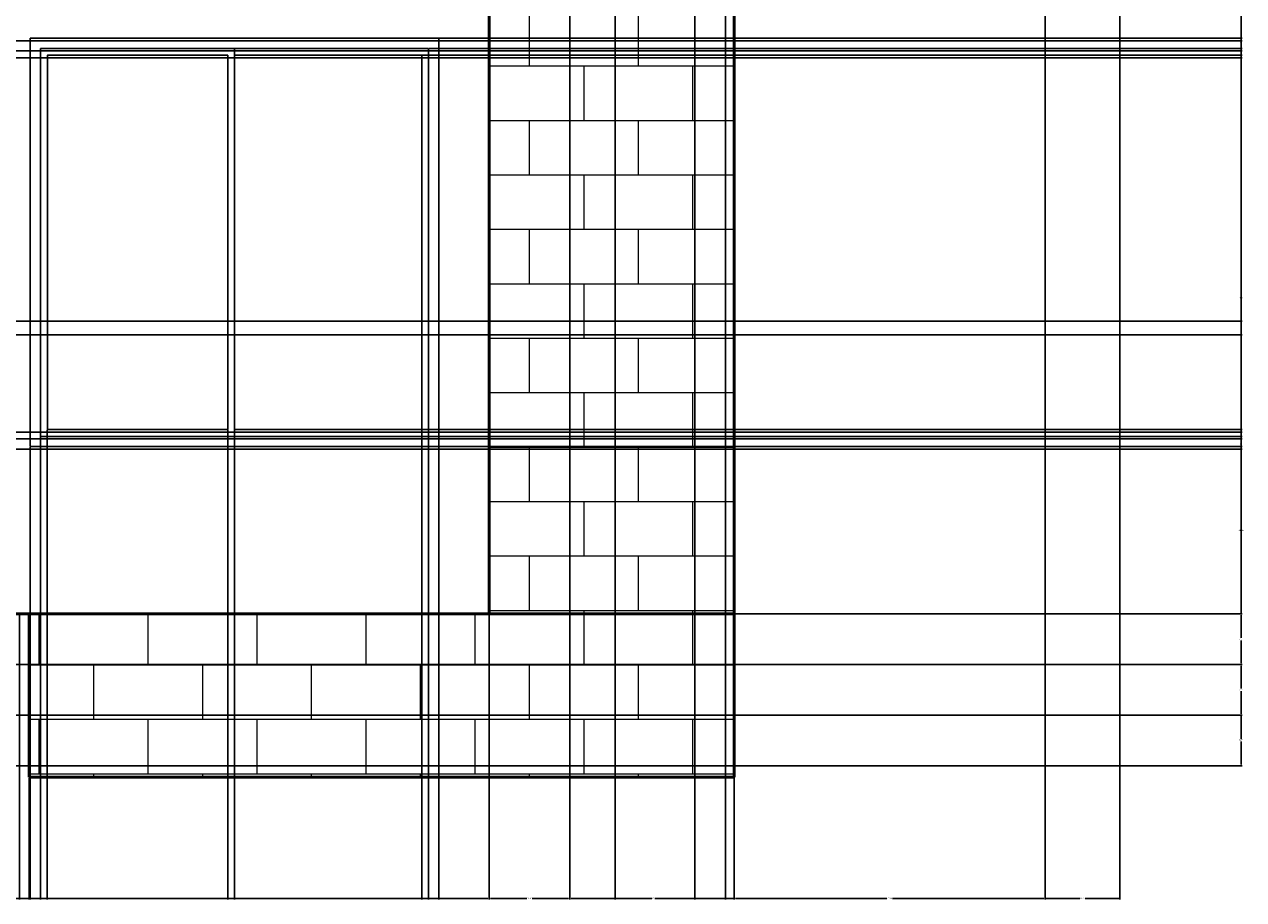
# Model space of a CAD drawing. Units: inches. Extents: x 27 to 409, y -26 to 294.
# Tile 5 of 7: x 230 to 409, y -26 to 102. Entities that reach past the tile are written whole.
import ezdxf

# ---------------------------------------------------------------- set-up
doc = ezdxf.new("R2010")
doc.units = ezdxf.units.IN
doc.header["$MEASUREMENT"] = 0
for name, color, linetype, lineweight in [('A-ANNO-DIMS', 2, 'Continuous', 18), ('A-FLOR-STRS', 2, 'Continuous', 25), ('A-GLAZ', 4, 'Continuous', 25), ('A-WALL', 7, 'Continuous', 50), ('A-WALL-PATT', 8, 'Continuous', 13)]:
    doc.layers.add(name, color=color, linetype=linetype, lineweight=lineweight)
doc.styles.get("Standard").update_dxf_attribs({"font": 'arial.ttf'})
doc.dimstyles.get("Standard").update_dxf_attribs({"dimtxt": 0.18, "dimasz": 0.18, "dimexe": 0.18, "dimexo": 0.0625, "dimgap": 0.09, "dimtad": 0, "dimtih": 1, "dimtoh": 1, "dimdec": 4, "dimzin": 0, "dimdsep": 46, "dimtxsty": 'Standard', "dimcen": 0.09, "dimadec": 0, "dimazin": 0, "dimtfac": 1, "dimtdec": 4, "dimtofl": 0, "dimtmove": 0, "dimatfit": 3, "dimfxl": 1, "dimtolj": 1, "dimtzin": 0, "dimarcsym": 0})

# ---------------------------------------------------------------- blocks, each defined once
blk = doc.blocks.new('*U6')
for p, q in [((1.5, 1.5), (1.5, 58.5)), ((1.5, 58.5), (30, 58.5)), ((30, 1.5), (30, 58.5)), ((30, 58.5), (58.5, 58.5)), ((58.5, 58.5), (58.5, 1.5)), ((30, 1.5), (1.5, 1.5)), ((58.5, 1.5), (30, 1.5))]:
    blk.add_line(p, q)
blk.add_lwpolyline([(0, 0), (0, 60), (60, 60), (60, 0)], close=True)
for points in [[(29, 57.5), (29, 2.5), (2.5, 2.5), (2.5, 57.5), (29, 57.5)], [(30, 57.5), (57.5, 57.5), (57.5, 2.5), (30, 2.5)]]:
    blk.add_lwpolyline(points)
blk = doc.blocks.new('*D20')
at = {"layer": 'A-ANNO-DIMS', "color": 0, "lineweight": -2, "transparency": 16777216}
for p, q in [((210.09, 143.71), (210.09, -26.5)), ((230.52, -8.58), (230.52, -26.5)), ((210.27, -26.32), (219.84, -26.32)), ((230.34, -26.32), (220.77, -26.32))]:
    blk.add_line(p, q, dxfattribs=at)
at = {"layer": 'A-ANNO-DIMS', "color": 0, "transparency": 16777216}
for points in [[(210.27, -26.29), (210.27, -26.35), (210.09, -26.32)], [(230.34, -26.29), (230.34, -26.35), (230.52, -26.32)]]:
    blk.add_solid(points, dxfattribs=at)
at = {"layer": 'Defpoints', "color": 0, "transparency": 16777216}
for p in [(210.09, 143.77), (230.52, -8.52), (230.52, -26.32)]:
    blk.add_point(p, dxfattribs=at)
at = {"layer": 'A-ANNO-DIMS', "color": 0, "transparency": 16777216, "insert": (220.31, -26.32), "char_height": 0.18, "attachment_point": 5}
blk.add_mtext('\\A1;20.435', dxfattribs=at)
blk = doc.blocks.new('*D21')
at = {"layer": 'A-ANNO-DIMS', "color": 0, "lineweight": -2, "transparency": 16777216}
for p, q in [((298.08, 108.32), (298.08, -26.5)), ((230.52, -8.58), (230.52, -26.5)), ((230.7, -26.32), (263.9, -26.32)), ((297.9, -26.32), (264.69, -26.32))]:
    blk.add_line(p, q, dxfattribs=at)
at = {"layer": 'A-ANNO-DIMS', "color": 0, "transparency": 16777216}
for points in [[(230.7, -26.29), (230.7, -26.35), (230.52, -26.32)], [(297.9, -26.29), (297.9, -26.35), (298.08, -26.32)]]:
    blk.add_solid(points, dxfattribs=at)
at = {"layer": 'Defpoints', "color": 0, "transparency": 16777216}
for p in [(298.08, 108.38), (230.52, -8.52), (298.08, -26.32)]:
    blk.add_point(p, dxfattribs=at)
at = {"layer": 'A-ANNO-DIMS', "color": 0, "transparency": 16777216, "insert": (264.3, -26.32), "char_height": 0.18, "attachment_point": 5}
blk.add_mtext('\\A1;67.55', dxfattribs=at)
blk = doc.blocks.new('*D22')
at = {"layer": 'A-ANNO-DIMS', "color": 0, "lineweight": -2, "transparency": 16777216}
for p, q in [((309.93, 158.34), (309.93, -26.5)), ((298.08, 108.32), (298.08, -26.5)), ((298.26, -26.32), (303.61, -26.32)), ((309.75, -26.32), (304.39, -26.32))]:
    blk.add_line(p, q, dxfattribs=at)
at = {"layer": 'A-ANNO-DIMS', "color": 0, "transparency": 16777216}
for points in [[(298.26, -26.29), (298.26, -26.35), (298.08, -26.32)], [(309.75, -26.29), (309.75, -26.35), (309.93, -26.32)]]:
    blk.add_solid(points, dxfattribs=at)
at = {"layer": 'Defpoints', "color": 0, "transparency": 16777216}
for p in [(309.93, 158.4), (298.08, 108.38), (309.93, -26.32)]:
    blk.add_point(p, dxfattribs=at)
at = {"layer": 'A-ANNO-DIMS', "color": 0, "transparency": 16777216, "insert": (304, -26.32), "char_height": 0.18, "attachment_point": 5}
blk.add_mtext('\\A1;11.85', dxfattribs=at)
blk = doc.blocks.new('*D23')
at = {"layer": 'A-ANNO-DIMS', "color": 0, "lineweight": -2, "transparency": 16777216}
for p, q in [((309.93, 158.34), (309.93, -26.5)), ((334.08, 15.42), (334.08, -26.5)), ((310.11, -26.32), (321.6, -26.32)), ((333.9, -26.32), (322.4, -26.32))]:
    blk.add_line(p, q, dxfattribs=at)
at = {"layer": 'A-ANNO-DIMS', "color": 0, "transparency": 16777216}
for points in [[(310.11, -26.29), (310.11, -26.35), (309.93, -26.32)], [(333.9, -26.29), (333.9, -26.35), (334.08, -26.32)]]:
    blk.add_solid(points, dxfattribs=at)
at = {"layer": 'Defpoints', "color": 0, "transparency": 16777216}
for p in [(309.93, 158.4), (334.08, 15.48), (334.08, -26.32)]:
    blk.add_point(p, dxfattribs=at)
at = {"layer": 'A-ANNO-DIMS', "color": 0, "transparency": 16777216, "insert": (322, -26.32), "char_height": 0.18, "attachment_point": 5}
blk.add_mtext('\\A1;24.15', dxfattribs=at)
blk = doc.blocks.new('*D24')
at = {"layer": 'A-ANNO-DIMS', "color": 0, "lineweight": -2, "transparency": 16777216}
for p, q in [((379.72, 117.44), (379.72, -26.5)), ((334.08, 15.42), (334.08, -26.5)), ((334.26, -26.32), (356.5, -26.32)), ((379.54, -26.32), (357.29, -26.32))]:
    blk.add_line(p, q, dxfattribs=at)
at = {"layer": 'A-ANNO-DIMS', "color": 0, "transparency": 16777216}
for points in [[(334.26, -26.29), (334.26, -26.35), (334.08, -26.32)], [(379.54, -26.29), (379.54, -26.35), (379.72, -26.32)]]:
    blk.add_solid(points, dxfattribs=at)
at = {"layer": 'Defpoints', "color": 0, "transparency": 16777216}
for p in [(379.72, 117.5), (334.08, 15.48), (379.72, -26.32)]:
    blk.add_point(p, dxfattribs=at)
at = {"layer": 'A-ANNO-DIMS', "color": 0, "transparency": 16777216, "insert": (356.9, -26.32), "char_height": 0.18, "attachment_point": 5}
blk.add_mtext('\\A1;45.64', dxfattribs=at)
blk = doc.blocks.new('*D25')
at = {"layer": 'A-ANNO-DIMS', "color": 0, "lineweight": -2, "transparency": 16777216}
for p, q in [((390.71, 136.19), (390.71, -26.5)), ((379.72, 117.44), (379.72, -26.5)), ((379.9, -26.32), (384.83, -26.32)), ((390.53, -26.32), (385.6, -26.32))]:
    blk.add_line(p, q, dxfattribs=at)
at = {"layer": 'A-ANNO-DIMS', "color": 0, "transparency": 16777216}
for points in [[(379.9, -26.29), (379.9, -26.35), (379.72, -26.32)], [(390.53, -26.29), (390.53, -26.35), (390.71, -26.32)]]:
    blk.add_solid(points, dxfattribs=at)
at = {"layer": 'Defpoints', "color": 0, "transparency": 16777216}
for p in [(390.71, 136.26), (379.72, 117.5), (390.71, -26.32)]:
    blk.add_point(p, dxfattribs=at)
at = {"layer": 'A-ANNO-DIMS', "color": 0, "transparency": 16777216, "insert": (385.21, -26.32), "char_height": 0.18, "attachment_point": 5}
blk.add_mtext('\\A1;10.99', dxfattribs=at)
blk = doc.blocks.new('*D39')
at = {"layer": 'A-ANNO-DIMS', "color": 0, "lineweight": -2, "transparency": 16777216}
for p, q in [((230.59, 0.62), (408.69, 0.62)), ((408.51, 0.44), (408.51, -2.92)), ((408.51, -6.64), (408.51, -3.28)), ((230.59, -6.82), (408.69, -6.82))]:
    blk.add_line(p, q, dxfattribs=at)
at = {"layer": 'A-ANNO-DIMS', "color": 0, "transparency": 16777216}
for points in [[(408.48, 0.44), (408.54, 0.44), (408.51, 0.62)], [(408.48, -6.64), (408.54, -6.64), (408.51, -6.82)]]:
    blk.add_solid(points, dxfattribs=at)
at = {"layer": 'Defpoints', "color": 0, "transparency": 16777216}
for p in [(230.52, 0.62), (408.51, 0.62), (230.52, -6.82)]:
    blk.add_point(p, dxfattribs=at)
at = {"layer": 'A-ANNO-DIMS', "color": 0, "transparency": 16777216, "insert": (408.51, -3.1), "char_height": 0.18, "attachment_point": 5}
blk.add_mtext('\\A1;7.433', dxfattribs=at)
blk = doc.blocks.new('*D40')
at = {"layer": 'A-ANNO-DIMS', "color": 0, "lineweight": -2, "transparency": 16777216}
for p, q in [((230.59, 8.05), (408.69, 8.05)), ((408.51, 7.87), (408.51, 4.51)), ((408.51, 0.8), (408.51, 4.15)), ((230.59, 0.62), (408.69, 0.62))]:
    blk.add_line(p, q, dxfattribs=at)
at = {"layer": 'A-ANNO-DIMS', "color": 0, "transparency": 16777216}
for points in [[(408.48, 7.87), (408.54, 7.87), (408.51, 8.05)], [(408.48, 0.8), (408.54, 0.8), (408.51, 0.62)]]:
    blk.add_solid(points, dxfattribs=at)
at = {"layer": 'Defpoints', "color": 0, "transparency": 16777216}
for p in [(230.52, 8.05), (408.51, 8.05), (230.52, 0.62)]:
    blk.add_point(p, dxfattribs=at)
at = {"layer": 'A-ANNO-DIMS', "color": 0, "transparency": 16777216, "insert": (408.51, 4.33), "char_height": 0.18, "attachment_point": 5}
blk.add_mtext('\\A1;7.433', dxfattribs=at)
blk = doc.blocks.new('*D41')
at = {"layer": 'A-ANNO-DIMS', "color": 0, "lineweight": -2, "transparency": 16777216}
for p, q in [((334.14, 15.48), (408.69, 15.48)), ((408.51, 15.3), (408.51, 11.95)), ((408.51, 8.23), (408.51, 11.58)), ((230.59, 8.05), (408.69, 8.05))]:
    blk.add_line(p, q, dxfattribs=at)
at = {"layer": 'A-ANNO-DIMS', "color": 0, "transparency": 16777216}
for points in [[(408.48, 15.3), (408.54, 15.3), (408.51, 15.48)], [(408.48, 8.23), (408.54, 8.23), (408.51, 8.05)]]:
    blk.add_solid(points, dxfattribs=at)
at = {"layer": 'Defpoints', "color": 0, "transparency": 16777216}
for p in [(334.08, 15.48), (408.51, 15.48), (230.52, 8.05)]:
    blk.add_point(p, dxfattribs=at)
at = {"layer": 'A-ANNO-DIMS', "color": 0, "transparency": 16777216, "insert": (408.51, 11.77), "char_height": 0.18, "attachment_point": 5}
blk.add_mtext('\\A1;7.433', dxfattribs=at)
blk = doc.blocks.new('*D42')
at = {"layer": 'A-ANNO-DIMS', "color": 0, "lineweight": -2, "transparency": 16777216}
for p, q in [((334.14, 108.38), (408.69, 108.38)), ((408.51, 108.2), (408.51, 62.11)), ((408.51, 15.66), (408.51, 61.75)), ((334.14, 15.48), (408.69, 15.48))]:
    blk.add_line(p, q, dxfattribs=at)
at = {"layer": 'A-ANNO-DIMS', "color": 0, "transparency": 16777216}
for points in [[(408.48, 108.2), (408.54, 108.2), (408.51, 108.38)], [(408.48, 15.66), (408.54, 15.66), (408.51, 15.48)]]:
    blk.add_solid(points, dxfattribs=at)
at = {"layer": 'Defpoints', "color": 0, "transparency": 16777216}
for p in [(334.08, 108.38), (408.51, 108.38), (334.08, 15.48)]:
    blk.add_point(p, dxfattribs=at)
at = {"layer": 'A-ANNO-DIMS', "color": 0, "transparency": 16777216, "insert": (408.51, 61.93), "char_height": 0.18, "attachment_point": 5}
blk.add_mtext('\\A1;92.9', dxfattribs=at)
blk = doc.blocks.new('*D60')
at = {"layer": 'A-ANNO-DIMS', "color": 0, "lineweight": -2, "transparency": 16777216}
for p, q in [((230.68, 40), (230.68, -26.5)), ((229.1, 15.43), (229.1, -26.5)), ((229.28, -26.32), (229.53, -26.32)), ((230.5, -26.32), (230.26, -26.32))]:
    blk.add_line(p, q, dxfattribs=at)
at = {"layer": 'A-ANNO-DIMS', "color": 0, "transparency": 16777216}
for points in [[(229.28, -26.29), (229.28, -26.35), (229.1, -26.32)], [(230.5, -26.29), (230.5, -26.35), (230.68, -26.32)]]:
    blk.add_solid(points, dxfattribs=at)
at = {"layer": 'Defpoints', "color": 0, "transparency": 16777216}
for p in [(230.68, 40.07), (229.1, 15.5), (230.68, -26.32)]:
    blk.add_point(p, dxfattribs=at)
at = {"layer": 'A-ANNO-DIMS', "color": 0, "transparency": 16777216, "insert": (229.89, -26.32), "char_height": 0.18, "attachment_point": 5}
blk.add_mtext('\\A1;1.581', dxfattribs=at)
blk = doc.blocks.new('*D61')
at = {"layer": 'A-ANNO-DIMS', "color": 0, "lineweight": -2, "transparency": 16777216}
for p, q in [((232.18, 41.5), (232.18, -26.5)), ((230.68, 40), (230.68, -26.5)), ((230.86, -26.32), (231.19, -26.32)), ((232, -26.32), (231.68, -26.32))]:
    blk.add_line(p, q, dxfattribs=at)
at = {"layer": 'A-ANNO-DIMS', "color": 0, "transparency": 16777216}
for points in [[(230.86, -26.29), (230.86, -26.35), (230.68, -26.32)], [(232, -26.29), (232, -26.35), (232.18, -26.32)]]:
    blk.add_solid(points, dxfattribs=at)
at = {"layer": 'Defpoints', "color": 0, "transparency": 16777216}
for p in [(232.18, 41.57), (230.68, 40.07), (232.18, -26.32)]:
    blk.add_point(p, dxfattribs=at)
at = {"layer": 'A-ANNO-DIMS', "color": 0, "transparency": 16777216, "insert": (231.43, -26.32), "char_height": 0.18, "attachment_point": 5}
blk.add_mtext('\\A1;1.5', dxfattribs=at)
blk = doc.blocks.new('*D62')
at = {"layer": 'A-ANNO-DIMS', "color": 0, "lineweight": -2, "transparency": 16777216}
for p, q in [((232.18, 41.5), (232.18, -26.5)), ((233.18, 42.5), (233.18, -26.5)), ((232.36, -26.32), (232.56, -26.32)), ((233, -26.32), (232.81, -26.32))]:
    blk.add_line(p, q, dxfattribs=at)
at = {"layer": 'A-ANNO-DIMS', "color": 0, "transparency": 16777216}
for points in [[(232.36, -26.29), (232.36, -26.35), (232.18, -26.32)], [(233, -26.29), (233, -26.35), (233.18, -26.32)]]:
    blk.add_solid(points, dxfattribs=at)
at = {"layer": 'Defpoints', "color": 0, "transparency": 16777216}
for p in [(232.18, 41.57), (233.18, 42.57), (233.18, -26.32)]:
    blk.add_point(p, dxfattribs=at)
at = {"layer": 'A-ANNO-DIMS', "color": 0, "transparency": 16777216, "insert": (232.68, -26.32), "char_height": 0.18, "attachment_point": 5}
blk.add_mtext('\\A1;1', dxfattribs=at)
blk = doc.blocks.new('*D63')
at = {"layer": 'A-ANNO-DIMS', "color": 0, "lineweight": -2, "transparency": 16777216}
for p, q in [((233.18, 42.5), (233.18, -26.5)), ((259.68, 42.5), (259.68, -26.5)), ((233.36, -26.32), (246.11, -26.32)), ((259.5, -26.32), (246.76, -26.32))]:
    blk.add_line(p, q, dxfattribs=at)
at = {"layer": 'A-ANNO-DIMS', "color": 0, "transparency": 16777216}
for points in [[(233.36, -26.29), (233.36, -26.35), (233.18, -26.32)], [(259.5, -26.29), (259.5, -26.35), (259.68, -26.32)]]:
    blk.add_solid(points, dxfattribs=at)
at = {"layer": 'Defpoints', "color": 0, "transparency": 16777216}
for p in [(233.18, 42.57), (259.68, 42.57), (259.68, -26.32)]:
    blk.add_point(p, dxfattribs=at)
at = {"layer": 'A-ANNO-DIMS', "color": 0, "transparency": 16777216, "insert": (246.43, -26.32), "char_height": 0.18, "attachment_point": 5}
blk.add_mtext('\\A1;26.5', dxfattribs=at)
blk = doc.blocks.new('*D64')
at = {"layer": 'A-ANNO-DIMS', "color": 0, "lineweight": -2, "transparency": 16777216}
for p, q in [((259.68, 42.5), (259.68, -26.5)), ((260.68, 41.5), (260.68, -26.5)), ((259.86, -26.32), (260.06, -26.32)), ((260.5, -26.32), (260.31, -26.32))]:
    blk.add_line(p, q, dxfattribs=at)
at = {"layer": 'A-ANNO-DIMS', "color": 0, "transparency": 16777216}
for points in [[(259.86, -26.29), (259.86, -26.35), (259.68, -26.32)], [(260.5, -26.29), (260.5, -26.35), (260.68, -26.32)]]:
    blk.add_solid(points, dxfattribs=at)
at = {"layer": 'Defpoints', "color": 0, "transparency": 16777216}
for p in [(259.68, 42.57), (260.68, 41.57), (260.68, -26.32)]:
    blk.add_point(p, dxfattribs=at)
at = {"layer": 'A-ANNO-DIMS', "color": 0, "transparency": 16777216, "insert": (260.18, -26.32), "char_height": 0.18, "attachment_point": 5}
blk.add_mtext('\\A1;1', dxfattribs=at)
blk = doc.blocks.new('*D65')
at = {"layer": 'A-ANNO-DIMS', "color": 0, "lineweight": -2, "transparency": 16777216}
for p, q in [((260.68, 41.5), (260.68, -26.5)), ((288.18, 42.5), (288.18, -26.5)), ((260.86, -26.32), (274.11, -26.32)), ((288, -26.32), (274.76, -26.32))]:
    blk.add_line(p, q, dxfattribs=at)
at = {"layer": 'A-ANNO-DIMS', "color": 0, "transparency": 16777216}
for points in [[(260.86, -26.29), (260.86, -26.35), (260.68, -26.32)], [(288, -26.29), (288, -26.35), (288.18, -26.32)]]:
    blk.add_solid(points, dxfattribs=at)
at = {"layer": 'Defpoints', "color": 0, "transparency": 16777216}
for p in [(260.68, 41.57), (288.18, 42.57), (288.18, -26.32)]:
    blk.add_point(p, dxfattribs=at)
at = {"layer": 'A-ANNO-DIMS', "color": 0, "transparency": 16777216, "insert": (274.43, -26.32), "char_height": 0.18, "attachment_point": 5}
blk.add_mtext('\\A1;27.5', dxfattribs=at)
blk = doc.blocks.new('*D66')
at = {"layer": 'A-ANNO-DIMS', "color": 0, "lineweight": -2, "transparency": 16777216}
for p, q in [((288.18, 42.5), (288.18, -26.5)), ((289.18, 41.5), (289.18, -26.5)), ((288.36, -26.32), (288.56, -26.32)), ((289, -26.32), (288.81, -26.32))]:
    blk.add_line(p, q, dxfattribs=at)
at = {"layer": 'A-ANNO-DIMS', "color": 0, "transparency": 16777216}
for points in [[(288.36, -26.29), (288.36, -26.35), (288.18, -26.32)], [(289, -26.29), (289, -26.35), (289.18, -26.32)]]:
    blk.add_solid(points, dxfattribs=at)
at = {"layer": 'Defpoints', "color": 0, "transparency": 16777216}
for p in [(288.18, 42.57), (289.18, 41.57), (289.18, -26.32)]:
    blk.add_point(p, dxfattribs=at)
at = {"layer": 'A-ANNO-DIMS', "color": 0, "transparency": 16777216, "insert": (288.68, -26.32), "char_height": 0.18, "attachment_point": 5}
blk.add_mtext('\\A1;1', dxfattribs=at)
blk = doc.blocks.new('*D67')
at = {"layer": 'A-ANNO-DIMS', "color": 0, "lineweight": -2, "transparency": 16777216}
for p, q in [((289.18, 41.5), (289.18, -26.5)), ((290.68, 40), (290.68, -26.5)), ((289.36, -26.32), (289.69, -26.32)), ((290.5, -26.32), (290.18, -26.32))]:
    blk.add_line(p, q, dxfattribs=at)
at = {"layer": 'A-ANNO-DIMS', "color": 0, "transparency": 16777216}
for points in [[(289.36, -26.29), (289.36, -26.35), (289.18, -26.32)], [(290.5, -26.29), (290.5, -26.35), (290.68, -26.32)]]:
    blk.add_solid(points, dxfattribs=at)
at = {"layer": 'Defpoints', "color": 0, "transparency": 16777216}
for p in [(289.18, 41.57), (290.68, 40.07), (290.68, -26.32)]:
    blk.add_point(p, dxfattribs=at)
at = {"layer": 'A-ANNO-DIMS', "color": 0, "transparency": 16777216, "insert": (289.93, -26.32), "char_height": 0.18, "attachment_point": 5}
blk.add_mtext('\\A1;1.5', dxfattribs=at)
blk = doc.blocks.new('*D68')
at = {"layer": 'A-ANNO-DIMS', "color": 0, "lineweight": -2, "transparency": 16777216}
for p, q in [((290.68, 40), (290.68, -26.5)), ((298.08, 15.42), (298.08, -26.5)), ((290.86, -26.32), (294.06, -26.32)), ((297.9, -26.32), (294.7, -26.32))]:
    blk.add_line(p, q, dxfattribs=at)
at = {"layer": 'A-ANNO-DIMS', "color": 0, "transparency": 16777216}
for points in [[(290.86, -26.29), (290.86, -26.35), (290.68, -26.32)], [(297.9, -26.29), (297.9, -26.35), (298.08, -26.32)]]:
    blk.add_solid(points, dxfattribs=at)
at = {"layer": 'Defpoints', "color": 0, "transparency": 16777216}
for p in [(290.68, 40.07), (298.08, 15.48), (298.08, -26.32)]:
    blk.add_point(p, dxfattribs=at)
at = {"layer": 'A-ANNO-DIMS', "color": 0, "transparency": 16777216, "insert": (294.38, -26.32), "char_height": 0.18, "attachment_point": 5}
blk.add_mtext('\\A1;7.39', dxfattribs=at)
blk = doc.blocks.new('*D74')
at = {"layer": 'A-ANNO-DIMS', "color": 0, "lineweight": -2, "transparency": 16777216}
for p, q in [((224.17, 56.5), (408.69, 56.5)), ((408.51, 56.32), (408.51, 36.18)), ((408.51, 15.68), (408.51, 35.81)), ((226.17, 15.5), (408.69, 15.5))]:
    blk.add_line(p, q, dxfattribs=at)
at = {"layer": 'A-ANNO-DIMS', "color": 0, "transparency": 16777216}
for points in [[(408.48, 56.32), (408.54, 56.32), (408.51, 56.5)], [(408.48, 15.68), (408.54, 15.68), (408.51, 15.5)]]:
    blk.add_solid(points, dxfattribs=at)
at = {"layer": 'Defpoints', "color": 0, "transparency": 16777216}
for p in [(224.1, 56.5), (408.51, 56.5), (226.1, 15.5)]:
    blk.add_point(p, dxfattribs=at)
at = {"layer": 'A-ANNO-DIMS', "color": 0, "transparency": 16777216, "insert": (408.51, 36), "char_height": 0.18, "attachment_point": 5}
blk.add_mtext('\\A1;41', dxfattribs=at)
blk = doc.blocks.new('*D75')
at = {"layer": 'A-ANNO-DIMS', "color": 0, "lineweight": -2, "transparency": 16777216}
for p, q in [((224.17, 58.5), (408.69, 58.5)), ((408.51, 58.32), (408.51, 57.68)), ((408.51, 56.68), (408.51, 57.31)), ((224.17, 56.5), (408.69, 56.5))]:
    blk.add_line(p, q, dxfattribs=at)
at = {"layer": 'A-ANNO-DIMS', "color": 0, "transparency": 16777216}
for points in [[(408.48, 58.32), (408.54, 58.32), (408.51, 58.5)], [(408.48, 56.68), (408.54, 56.68), (408.51, 56.5)]]:
    blk.add_solid(points, dxfattribs=at)
at = {"layer": 'Defpoints', "color": 0, "transparency": 16777216}
for p in [(224.1, 58.5), (408.51, 58.5), (224.1, 56.5)]:
    blk.add_point(p, dxfattribs=at)
at = {"layer": 'A-ANNO-DIMS', "color": 0, "transparency": 16777216, "insert": (408.51, 57.5), "char_height": 0.18, "attachment_point": 5}
blk.add_mtext('\\A1;2', dxfattribs=at)
blk = doc.blocks.new('*D76')
at = {"layer": 'A-ANNO-DIMS', "color": 0, "lineweight": -2, "transparency": 16777216}
for p, q in [((290.75, 40.07), (408.69, 40.07)), ((408.51, 39.89), (408.51, 27.96)), ((408.51, 15.66), (408.51, 27.59)), ((298.14, 15.48), (408.69, 15.48))]:
    blk.add_line(p, q, dxfattribs=at)
at = {"layer": 'A-ANNO-DIMS', "color": 0, "transparency": 16777216}
for points in [[(408.48, 39.89), (408.54, 39.89), (408.51, 40.07)], [(408.48, 15.66), (408.54, 15.66), (408.51, 15.48)]]:
    blk.add_solid(points, dxfattribs=at)
at = {"layer": 'Defpoints', "color": 0, "transparency": 16777216}
for p in [(290.68, 40.07), (408.51, 40.07), (298.08, 15.48)]:
    blk.add_point(p, dxfattribs=at)
at = {"layer": 'A-ANNO-DIMS', "color": 0, "transparency": 16777216, "insert": (408.51, 27.77), "char_height": 0.18, "attachment_point": 5}
blk.add_mtext('\\A1;24.585', dxfattribs=at)
blk = doc.blocks.new('*D77')
at = {"layer": 'A-ANNO-DIMS', "color": 0, "lineweight": -2, "transparency": 16777216}
for p, q in [((289.25, 41.57), (408.69, 41.57)), ((408.51, 41.39), (408.51, 41)), ((290.75, 40.07), (408.69, 40.07)), ((408.51, 40.25), (408.51, 40.64))]:
    blk.add_line(p, q, dxfattribs=at)
at = {"layer": 'A-ANNO-DIMS', "color": 0, "transparency": 16777216}
for points in [[(408.48, 41.39), (408.54, 41.39), (408.51, 41.57)], [(408.48, 40.25), (408.54, 40.25), (408.51, 40.07)]]:
    blk.add_solid(points, dxfattribs=at)
at = {"layer": 'Defpoints', "color": 0, "transparency": 16777216}
for p in [(289.18, 41.57), (408.51, 41.57), (290.68, 40.07)]:
    blk.add_point(p, dxfattribs=at)
at = {"layer": 'A-ANNO-DIMS', "color": 0, "transparency": 16777216, "insert": (408.51, 40.82), "char_height": 0.18, "attachment_point": 5}
blk.add_mtext('\\A1;1.5', dxfattribs=at)
blk = doc.blocks.new('*D78')
at = {"layer": 'A-ANNO-DIMS', "color": 0, "lineweight": -2, "transparency": 16777216}
for p, q in [((288.25, 42.57), (408.69, 42.57)), ((289.25, 41.57), (408.69, 41.57)), ((408.51, 42.39), (408.51, 42.25)), ((408.51, 41.75), (408.51, 41.89))]:
    blk.add_line(p, q, dxfattribs=at)
at = {"layer": 'A-ANNO-DIMS', "color": 0, "transparency": 16777216}
for points in [[(408.48, 42.39), (408.54, 42.39), (408.51, 42.57)], [(408.48, 41.75), (408.54, 41.75), (408.51, 41.57)]]:
    blk.add_solid(points, dxfattribs=at)
at = {"layer": 'Defpoints', "color": 0, "transparency": 16777216}
for p in [(288.18, 42.57), (289.18, 41.57), (408.51, 42.57)]:
    blk.add_point(p, dxfattribs=at)
at = {"layer": 'A-ANNO-DIMS', "color": 0, "transparency": 16777216, "insert": (408.51, 42.07), "char_height": 0.18, "attachment_point": 5}
blk.add_mtext('\\A1;1', dxfattribs=at)
blk = doc.blocks.new('*D79')
at = {"layer": 'A-ANNO-DIMS', "color": 0, "lineweight": -2, "transparency": 16777216}
for p, q in [((288.25, 97.57), (408.69, 97.57)), ((408.51, 97.39), (408.51, 70.25)), ((408.51, 42.75), (408.51, 69.89)), ((288.25, 42.57), (408.69, 42.57))]:
    blk.add_line(p, q, dxfattribs=at)
at = {"layer": 'A-ANNO-DIMS', "color": 0, "transparency": 16777216}
for points in [[(408.48, 97.39), (408.54, 97.39), (408.51, 97.57)], [(408.48, 42.75), (408.54, 42.75), (408.51, 42.57)]]:
    blk.add_solid(points, dxfattribs=at)
at = {"layer": 'Defpoints', "color": 0, "transparency": 16777216}
for p in [(288.18, 97.57), (408.51, 97.57), (288.18, 42.57)]:
    blk.add_point(p, dxfattribs=at)
at = {"layer": 'A-ANNO-DIMS', "color": 0, "transparency": 16777216, "insert": (408.51, 70.07), "char_height": 0.18, "attachment_point": 5}
blk.add_mtext('\\A1;55', dxfattribs=at)
blk = doc.blocks.new('*D80')
at = {"layer": 'A-ANNO-DIMS', "color": 0, "lineweight": -2, "transparency": 16777216}
for p, q in [((289.25, 98.57), (408.69, 98.57)), ((288.25, 97.57), (408.69, 97.57)), ((408.51, 98.39), (408.51, 98.25)), ((408.51, 97.75), (408.51, 97.89))]:
    blk.add_line(p, q, dxfattribs=at)
at = {"layer": 'A-ANNO-DIMS', "color": 0, "transparency": 16777216}
for points in [[(408.48, 98.39), (408.54, 98.39), (408.51, 98.57)], [(408.48, 97.75), (408.54, 97.75), (408.51, 97.57)]]:
    blk.add_solid(points, dxfattribs=at)
at = {"layer": 'Defpoints', "color": 0, "transparency": 16777216}
for p in [(289.18, 98.57), (408.51, 98.57), (288.18, 97.57)]:
    blk.add_point(p, dxfattribs=at)
at = {"layer": 'A-ANNO-DIMS', "color": 0, "transparency": 16777216, "insert": (408.51, 98.07), "char_height": 0.18, "attachment_point": 5}
blk.add_mtext('\\A1;1', dxfattribs=at)
blk = doc.blocks.new('*D81')
at = {"layer": 'A-ANNO-DIMS', "color": 0, "lineweight": -2, "transparency": 16777216}
for p, q in [((289.25, 98.57), (408.69, 98.57)), ((290.75, 100.07), (408.69, 100.07)), ((408.51, 99.89), (408.51, 99.5)), ((408.51, 98.75), (408.51, 99.14))]:
    blk.add_line(p, q, dxfattribs=at)
at = {"layer": 'A-ANNO-DIMS', "color": 0, "transparency": 16777216}
for points in [[(408.48, 99.89), (408.54, 99.89), (408.51, 100.07)], [(408.48, 98.75), (408.54, 98.75), (408.51, 98.57)]]:
    blk.add_solid(points, dxfattribs=at)
at = {"layer": 'Defpoints', "color": 0, "transparency": 16777216}
for p in [(289.18, 98.57), (290.68, 100.07), (408.51, 100.07)]:
    blk.add_point(p, dxfattribs=at)
at = {"layer": 'A-ANNO-DIMS', "color": 0, "transparency": 16777216, "insert": (408.51, 99.32), "char_height": 0.18, "attachment_point": 5}
blk.add_mtext('\\A1;1.5', dxfattribs=at)
blk = doc.blocks.new('*D82')
at = {"layer": 'A-ANNO-DIMS', "color": 0, "lineweight": -2, "transparency": 16777216}
for p, q in [((309.93, 228.32), (309.93, -26.5)), ((316.59, 228.32), (316.59, -26.5)), ((310.11, -26.32), (312.86, -26.32)), ((316.41, -26.32), (313.65, -26.32))]:
    blk.add_line(p, q, dxfattribs=at)
at = {"layer": 'A-ANNO-DIMS', "color": 0, "transparency": 16777216}
for points in [[(310.11, -26.29), (310.11, -26.35), (309.93, -26.32)], [(316.41, -26.29), (316.41, -26.35), (316.59, -26.32)]]:
    blk.add_solid(points, dxfattribs=at)
at = {"layer": 'Defpoints', "color": 0, "transparency": 16777216}
for p in [(309.93, 228.38), (316.59, 228.38), (316.59, -26.32)]:
    blk.add_point(p, dxfattribs=at)
at = {"layer": 'A-ANNO-DIMS', "color": 0, "transparency": 16777216, "insert": (313.26, -26.32), "char_height": 0.18, "attachment_point": 5}
blk.add_mtext('\\A1;6.665', dxfattribs=at)
blk = doc.blocks.new('*D83')
at = {"layer": 'A-ANNO-DIMS', "color": 0, "lineweight": -2, "transparency": 16777216}
for p, q in [((316.59, 228.32), (316.59, -26.5)), ((328.29, 228.32), (328.29, -26.5)), ((316.77, -26.32), (321.99, -26.32)), ((328.11, -26.32), (322.9, -26.32))]:
    blk.add_line(p, q, dxfattribs=at)
at = {"layer": 'A-ANNO-DIMS', "color": 0, "transparency": 16777216}
for points in [[(316.77, -26.29), (316.77, -26.35), (316.59, -26.32)], [(328.11, -26.29), (328.11, -26.35), (328.29, -26.32)]]:
    blk.add_solid(points, dxfattribs=at)
at = {"layer": 'Defpoints', "color": 0, "transparency": 16777216}
for p in [(316.59, 228.38), (328.29, 228.38), (328.29, -26.32)]:
    blk.add_point(p, dxfattribs=at)
at = {"layer": 'A-ANNO-DIMS', "color": 0, "transparency": 16777216, "insert": (322.44, -26.32), "char_height": 0.18, "attachment_point": 5}
blk.add_mtext('\\A1;11.699', dxfattribs=at)
blk = doc.blocks.new('*D84')
at = {"layer": 'A-ANNO-DIMS', "color": 0, "lineweight": -2, "transparency": 16777216}
for p, q in [((328.29, 228.32), (328.29, -26.5)), ((332.8, 228.32), (332.8, -26.5)), ((328.47, -26.32), (330.17, -26.32)), ((332.62, -26.32), (330.93, -26.32))]:
    blk.add_line(p, q, dxfattribs=at)
at = {"layer": 'A-ANNO-DIMS', "color": 0, "transparency": 16777216}
for points in [[(328.47, -26.29), (328.47, -26.35), (328.29, -26.32)], [(332.62, -26.29), (332.62, -26.35), (332.8, -26.32)]]:
    blk.add_solid(points, dxfattribs=at)
at = {"layer": 'Defpoints', "color": 0, "transparency": 16777216}
for p in [(328.29, 228.38), (332.8, 228.38), (332.8, -26.32)]:
    blk.add_point(p, dxfattribs=at)
at = {"layer": 'A-ANNO-DIMS', "color": 0, "transparency": 16777216, "insert": (330.55, -26.32), "char_height": 0.18, "attachment_point": 5}
blk.add_mtext('\\A1;4.511', dxfattribs=at)
blk = doc.blocks.new('*D108')
at = {"layer": 'A-ANNO-DIMS', "color": 0, "lineweight": -2, "transparency": 16777216}
for p, q in [((156.23, 41.21), (408.69, 41.21)), ((166.14, 39.71), (408.69, 39.71)), ((408.51, 41.03), (408.51, 40.64)), ((408.51, 39.89), (408.51, 40.28))]:
    blk.add_line(p, q, dxfattribs=at)
at = {"layer": 'A-ANNO-DIMS', "color": 0, "transparency": 16777216}
for points in [[(408.48, 41.03), (408.54, 41.03), (408.51, 41.21)], [(408.48, 39.89), (408.54, 39.89), (408.51, 39.71)]]:
    blk.add_solid(points, dxfattribs=at)
at = {"layer": 'Defpoints', "color": 0, "transparency": 16777216}
for p in [(156.17, 41.21), (408.51, 41.21), (166.08, 39.71)]:
    blk.add_point(p, dxfattribs=at)
at = {"layer": 'A-ANNO-DIMS', "color": 0, "transparency": 16777216, "insert": (408.51, 40.46), "char_height": 0.18, "attachment_point": 5}
blk.add_mtext('\\A1;1.5', dxfattribs=at)
blk = doc.blocks.new('*D109')
at = {"layer": 'A-ANNO-DIMS', "color": 0, "lineweight": -2, "transparency": 16777216}
for p, q in [((155.23, 42.21), (408.69, 42.21)), ((156.23, 41.21), (408.69, 41.21)), ((408.51, 42.03), (408.51, 41.89)), ((408.51, 41.39), (408.51, 41.53))]:
    blk.add_line(p, q, dxfattribs=at)
at = {"layer": 'A-ANNO-DIMS', "color": 0, "transparency": 16777216}
for points in [[(408.48, 42.03), (408.54, 42.03), (408.51, 42.21)], [(408.48, 41.39), (408.54, 41.39), (408.51, 41.21)]]:
    blk.add_solid(points, dxfattribs=at)
at = {"layer": 'Defpoints', "color": 0, "transparency": 16777216}
for p in [(155.17, 42.21), (156.17, 41.21), (408.51, 42.21)]:
    blk.add_point(p, dxfattribs=at)
at = {"layer": 'A-ANNO-DIMS', "color": 0, "transparency": 16777216, "insert": (408.51, 41.71), "char_height": 0.18, "attachment_point": 5}
blk.add_mtext('\\A1;1', dxfattribs=at)
blk = doc.blocks.new('*D110')
at = {"layer": 'A-ANNO-DIMS', "color": 0, "lineweight": -2, "transparency": 16777216}
for p, q in [((155.23, 97.21), (408.69, 97.21)), ((408.51, 97.03), (408.51, 69.89)), ((408.51, 42.39), (408.51, 69.53)), ((155.23, 42.21), (408.69, 42.21))]:
    blk.add_line(p, q, dxfattribs=at)
at = {"layer": 'A-ANNO-DIMS', "color": 0, "transparency": 16777216}
for points in [[(408.48, 97.03), (408.54, 97.03), (408.51, 97.21)], [(408.48, 42.39), (408.54, 42.39), (408.51, 42.21)]]:
    blk.add_solid(points, dxfattribs=at)
at = {"layer": 'Defpoints', "color": 0, "transparency": 16777216}
for p in [(155.17, 97.21), (408.51, 97.21), (155.17, 42.21)]:
    blk.add_point(p, dxfattribs=at)
at = {"layer": 'A-ANNO-DIMS', "color": 0, "transparency": 16777216, "insert": (408.51, 69.71), "char_height": 0.18, "attachment_point": 5}
blk.add_mtext('\\A1;55', dxfattribs=at)
blk = doc.blocks.new('*D111')
at = {"layer": 'A-ANNO-DIMS', "color": 0, "lineweight": -2, "transparency": 16777216}
for p, q in [((155.23, 97.21), (408.69, 97.21)), ((156.23, 98.21), (408.69, 98.21)), ((408.51, 98.03), (408.51, 97.89)), ((408.51, 97.39), (408.51, 97.53))]:
    blk.add_line(p, q, dxfattribs=at)
at = {"layer": 'A-ANNO-DIMS', "color": 0, "transparency": 16777216}
for points in [[(408.48, 98.03), (408.54, 98.03), (408.51, 98.21)], [(408.48, 97.39), (408.54, 97.39), (408.51, 97.21)]]:
    blk.add_solid(points, dxfattribs=at)
at = {"layer": 'Defpoints', "color": 0, "transparency": 16777216}
for p in [(155.17, 97.21), (156.17, 98.21), (408.51, 98.21)]:
    blk.add_point(p, dxfattribs=at)
at = {"layer": 'A-ANNO-DIMS', "color": 0, "transparency": 16777216, "insert": (408.51, 97.71), "char_height": 0.18, "attachment_point": 5}
blk.add_mtext('\\A1;1', dxfattribs=at)
blk = doc.blocks.new('*D112')
at = {"layer": 'A-ANNO-DIMS', "color": 0, "lineweight": -2, "transparency": 16777216}
for p, q in [((157.73, 99.71), (408.69, 99.71)), ((408.51, 99.53), (408.51, 99.14)), ((408.51, 98.39), (408.51, 98.78)), ((156.23, 98.21), (408.69, 98.21))]:
    blk.add_line(p, q, dxfattribs=at)
at = {"layer": 'A-ANNO-DIMS', "color": 0, "transparency": 16777216}
for points in [[(408.48, 99.53), (408.54, 99.53), (408.51, 99.71)], [(408.48, 98.39), (408.54, 98.39), (408.51, 98.21)]]:
    blk.add_solid(points, dxfattribs=at)
at = {"layer": 'Defpoints', "color": 0, "transparency": 16777216}
for p in [(157.67, 99.71), (408.51, 99.71), (156.17, 98.21)]:
    blk.add_point(p, dxfattribs=at)
at = {"layer": 'A-ANNO-DIMS', "color": 0, "transparency": 16777216, "insert": (408.51, 98.96), "char_height": 0.18, "attachment_point": 5}
blk.add_mtext('\\A1;1.5', dxfattribs=at)

msp = doc.modelspace()

# ---------------------------------------------------------------- hatches: boundary and pattern name
at = {"layer": 'A-WALL-PATT'}
h = msp.add_hatch(dxfattribs=at)
h.set_pattern_fill('AR-B816', color=256)
h.paths.add_polyline_path([(334.0751, 108.3803), (298.0751, 108.3803), (298.0751, 15.4825), (334.0751, 15.4825)])
h = msp.add_hatch(dxfattribs=at)
h.set_pattern_fill('AR-B816', color=256)
h.paths.add_polyline_path([(334.0751, 15.4825), (230.5245, 15.4825), (230.5245, -8.5175), (334.0751, -8.5175)])

# ---------------------------------------------------------------- linework, layer by layer
at = {"layer": 'A-FLOR-STRS'}
for points in [[(187.493, 15.4825), (230.5245, 15.4825), (230.5245, 8.0491), (187.493, 8.0491)], [(187.493, 8.0491), (230.5245, 8.0491), (230.5245, 0.6158), (187.493, 0.6158)], [(187.493, 0.6158), (230.5245, 0.6158), (230.5245, -6.8175), (187.493, -6.8175)]]:
    msp.add_lwpolyline(points, close=True, dxfattribs=at)
at = {"layer": 'A-WALL'}
for p, q in [((334.0751, -8.5175), (334.0751, 135.4825)), ((298.0751, 15.4825), (298.0751, 108.3803)), ((94.0751, 15.4825), (334.0751, 15.4825)), ((230.5245, 15.4825), (230.5245, -8.5175)), ((230.5245, -8.5175), (334.0751, -8.5175))]:
    msp.add_line(p, q, dxfattribs=at)

# ---------------------------------------------------------------- block references
at = {"layer": 'A-GLAZ'}
msp.add_blockref('*U6', (230.6845, 40.0674), dxfattribs=at)

# ---------------------------------------------------------------- dimensions: what is measured, and where the dimension line sits
at = {"layer": 'A-ANNO-DIMS'}
for base, p1, p2, override, picture, middle in [((316.5916, -26.3175), (309.9262, 228.3803), (316.5916, 228.3803), {"dimdec": 3, "dimlfac": 1, "dimrnd": 0, "dimzin": 0, "dimdsep": 46, "dimlunit": 2}, '*D82', (313.2589, -26.3175)), ((328.29013, -26.31755), (316.59157, 228.38031), (328.29013, 228.38031), {"dimdec": 3, "dimlfac": 1, "dimrnd": 0, "dimzin": 0, "dimdsep": 46, "dimlunit": 2}, '*D83', (322.44085, -26.31755)), ((332.8007, -26.3175), (328.2901, 228.3803), (332.8007, 228.3803), {"dimdec": 3, "dimlfac": 1, "dimrnd": 0, "dimzin": 0, "dimdsep": 46, "dimlunit": 2}, '*D84', (330.5454, -26.3175)), ((309.9262, -26.3175), (298.0751, 108.3803), (309.9262, 158.4006), {"dimdec": 2, "dimlfac": 1, "dimrnd": 0, "dimzin": 0, "dimdsep": 46, "dimlunit": 2}, '*D22', (304.0006, -26.3175)), ((334.0751, -26.3175), (309.9262, 158.4006), (334.0751, 15.4825), {"dimdec": 2, "dimlfac": 1, "dimrnd": 0, "dimzin": 0, "dimdsep": 46, "dimlunit": 2}, '*D23', (322.0006, -26.3175)), ((230.5245, -26.3175), (210.0897, 143.7732), (230.5245, -8.5175), {"dimdec": 3, "dimlfac": 1, "dimrnd": 0, "dimzin": 0, "dimdsep": 46, "dimlunit": 2}, '*D20', (220.3071, -26.3175)), ((390.7054, -26.3175), (379.7157, 117.5036), (390.7054, 136.2572), {"dimdec": 2, "dimlfac": 1, "dimrnd": 0, "dimzin": 0, "dimdsep": 46, "dimlunit": 2}, '*D25', (385.2106, -26.3175)), ((379.7157, -26.3175), (334.0751, 15.4825), (379.7157, 117.5036), {"dimdec": 2, "dimlfac": 1, "dimrnd": 0, "dimzin": 0, "dimdsep": 46, "dimlunit": 2}, '*D24', (356.8954, -26.3175)), ((298.0751, -26.3175), (230.5245, -8.5175), (298.0751, 108.3803), {"dimdec": 2, "dimlfac": 1, "dimrnd": 0, "dimzin": 0, "dimdsep": 46, "dimlunit": 2}, '*D21', (264.2998, -26.3175)), ((232.1845, -26.3175), (230.6845, 40.0674), (232.1845, 41.5674), {"dimdec": 1, "dimlfac": 1, "dimrnd": 0, "dimzin": 0, "dimdsep": 46, "dimlunit": 2}, '*D61', (231.4345, -26.3175)), ((233.1845, -26.3175), (232.1845, 41.5674), (233.1845, 42.5674), {"dimdec": 0, "dimlfac": 1, "dimrnd": 0, "dimzin": 0, "dimdsep": 46, "dimlunit": 2}, '*D62', (232.6845, -26.3175)), ((259.6845, -26.3175), (233.1845, 42.5674), (259.6845, 42.5674), {"dimdec": 1, "dimlfac": 1, "dimrnd": 0, "dimzin": 0, "dimdsep": 46, "dimlunit": 2}, '*D63', (246.4345, -26.3175)), ((260.6845, -26.3175), (259.6845, 42.5674), (260.6845, 41.5674), {"dimdec": 0, "dimlfac": 1, "dimrnd": 0, "dimzin": 0, "dimdsep": 46, "dimlunit": 2}, '*D64', (260.1845, -26.3175)), ((288.1845, -26.3175), (260.6845, 41.5674), (288.1845, 42.5674), {"dimdec": 1, "dimlfac": 1, "dimrnd": 0, "dimzin": 0, "dimdsep": 46, "dimlunit": 2}, '*D65', (274.4345, -26.3175)), ((289.1845, -26.3175), (288.1845, 42.5674), (289.1845, 41.5674), {"dimdec": 0, "dimlfac": 1, "dimrnd": 0, "dimzin": 0, "dimdsep": 46, "dimlunit": 2}, '*D66', (288.6845, -26.3175)), ((290.6845, -26.3175), (289.1845, 41.5674), (290.6845, 40.0674), {"dimdec": 1, "dimlfac": 1, "dimrnd": 0, "dimzin": 0, "dimdsep": 46, "dimlunit": 2}, '*D67', (289.9345, -26.3175)), ((230.6845, -26.3175), (229.1036, 15.4952), (230.6845, 40.0674), {"dimdec": 3, "dimlfac": 1, "dimrnd": 0, "dimzin": 0, "dimdsep": 46, "dimlunit": 2}, '*D60', (229.894, -26.3175)), ((298.0751, -26.3175), (290.6845, 40.0674), (298.0751, 15.4825), {"dimdec": 2, "dimlfac": 1, "dimrnd": 0, "dimzin": 0, "dimdsep": 46, "dimlunit": 2}, '*D68', (294.3798, -26.3175))]:
    dim = msp.add_linear_dim(base=base, p1=p1, p2=p2, dimstyle='Standard', override=override, dxfattribs=at)
    dim.commit()
    dim.dimension.update_dxf_attribs({"geometry": picture, "text_midpoint": middle})
for base, p1, p2, override, picture, middle in [((408.5054, 108.3803), (334.0751, 15.4825), (334.0751, 108.3803), {"dimdec": 1, "dimlfac": 1, "dimrnd": 0, "dimzin": 0, "dimdsep": 46, "dimlunit": 2}, '*D42', (408.5054, 61.9314)), ((408.5054, 99.7093), (156.1666, 98.2093), (157.6666, 99.7093), {"dimdec": 1, "dimlfac": 1, "dimrnd": 0, "dimzin": 0, "dimdsep": 46, "dimlunit": 2}, '*D112', (408.5054, 98.9593)), ((408.5054, 98.5674), (288.1845, 97.5674), (289.1845, 98.5674), {"dimdec": 0, "dimlfac": 1, "dimrnd": 0, "dimzin": 0, "dimdsep": 46, "dimlunit": 2}, '*D80', (408.5054, 98.0674)), ((408.5054, 100.0674), (289.1845, 98.5674), (290.6845, 100.0674), {"dimdec": 1, "dimlfac": 1, "dimrnd": 0, "dimzin": 0, "dimdsep": 46, "dimlunit": 2}, '*D81', (408.5054, 99.3174)), ((408.5054, 98.2093), (155.1666, 97.2093), (156.1666, 98.2093), {"dimdec": 0, "dimlfac": 1, "dimrnd": 0, "dimzin": 0, "dimdsep": 46, "dimlunit": 2}, '*D111', (408.5054, 97.7093)), ((408.5054, 97.2093), (155.1666, 42.2093), (155.1666, 97.2093), {"dimdec": 0, "dimlfac": 1, "dimrnd": 0, "dimzin": 0, "dimdsep": 46, "dimlunit": 2}, '*D110', (408.5054, 69.7093)), ((408.5054, 97.5674), (288.1845, 42.5674), (288.1845, 97.5674), {"dimdec": 0, "dimlfac": 1, "dimrnd": 0, "dimzin": 0, "dimdsep": 46, "dimlunit": 2}, '*D79', (408.5054, 70.0674)), ((408.5054, 58.4952), (224.1036, 56.4952), (224.1036, 58.4952), {"dimdec": 0, "dimlfac": 1, "dimrnd": 0, "dimzin": 0, "dimdsep": 46, "dimlunit": 2}, '*D75', (408.5054, 57.4952)), ((408.5054, 56.4952), (226.1036, 15.4952), (224.1036, 56.4952), {"dimdec": 0, "dimlfac": 1, "dimrnd": 0, "dimzin": 0, "dimdsep": 46, "dimlunit": 2}, '*D74', (408.5054, 35.9952)), ((408.5054, 42.2093), (156.1666, 41.2093), (155.1666, 42.2093), {"dimdec": 0, "dimlfac": 1, "dimrnd": 0, "dimzin": 0, "dimdsep": 46, "dimlunit": 2}, '*D109', (408.5054, 41.7093)), ((408.5054, 41.2093), (166.0751, 39.7093), (156.1666, 41.2093), {"dimdec": 1, "dimlfac": 1, "dimrnd": 0, "dimzin": 0, "dimdsep": 46, "dimlunit": 2}, '*D108', (408.5054, 40.4593)), ((408.5054, 42.5674), (289.1845, 41.5674), (288.1845, 42.5674), {"dimdec": 0, "dimlfac": 1, "dimrnd": 0, "dimzin": 0, "dimdsep": 46, "dimlunit": 2}, '*D78', (408.5054, 42.0674)), ((408.5054, 41.5674), (290.6845, 40.0674), (289.1845, 41.5674), {"dimdec": 1, "dimlfac": 1, "dimrnd": 0, "dimzin": 0, "dimdsep": 46, "dimlunit": 2}, '*D77', (408.5054, 40.8174)), ((408.5054, 40.0674), (298.0751, 15.4825), (290.6845, 40.0674), {"dimdec": 3, "dimlfac": 1, "dimrnd": 0, "dimzin": 0, "dimdsep": 46, "dimlunit": 2}, '*D76', (408.5054, 27.7749)), ((408.5054, 15.4825), (230.5245, 8.0491), (334.0751, 15.4825), {"dimdec": 3, "dimlfac": 1, "dimrnd": 0, "dimzin": 0, "dimdsep": 46, "dimlunit": 2}, '*D41', (408.5054, 11.7658)), ((408.5054, 8.0491), (230.5245, 0.6158), (230.5245, 8.0491), {"dimdec": 3, "dimlfac": 1, "dimrnd": 0, "dimzin": 0, "dimdsep": 46, "dimlunit": 2}, '*D40', (408.5054, 4.3325)), ((408.5054, 0.6158), (230.5245, -6.8175), (230.5245, 0.6158), {"dimdec": 3, "dimlfac": 1, "dimrnd": 0, "dimzin": 0, "dimdsep": 46, "dimlunit": 2}, '*D39', (408.5054, -3.1008))]:
    dim = msp.add_linear_dim(base=base, p1=p1, p2=p2, angle=90, dimstyle='Standard', override=override, dxfattribs=at)
    dim.commit()
    dim.dimension.update_dxf_attribs({"geometry": picture, "text_midpoint": middle})

doc.saveas('drawing.dxf')
